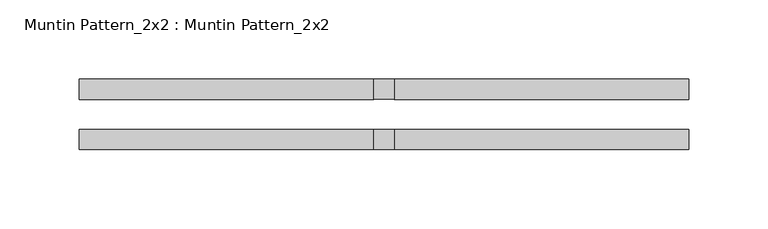
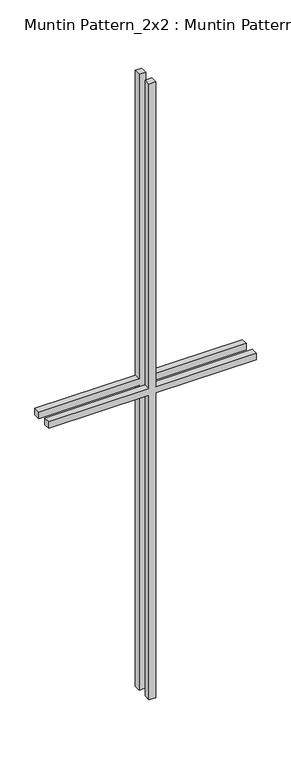
"""IFC4 building model written with IfcOpenShell, lengths in millimetres: proxy geometry, Muntin Pattern_2x2 : Muntin Pattern_2x2."""

from ifc_helpers import new_model, si_unit, frame, origin, place, context, project, spatial, polyline, outline, extrude, source, transform, mapped, element, save


def muntin_pattern_2x2_muntin_pattern_2x2_3dfd0a47(model_context):
    return source(origin(), model_context, "Body", "SweptSolid", [
        extrude(outline(polyline([(609.6, -6.35), (609.6, -192.0875), (596.9, -192.0875), (596.9, -6.35), (0.0, -6.35), (0.0, 6.35), (596.9, 6.35), (596.9, 192.0875), (609.6, 192.0875), (609.6, 6.35), (1206.5, 6.35), (1206.5, -6.35), (609.6, -6.35)])), frame((0.0, -22.225, 0.0), z_axis=(0.0, 1.0, 0.0), x_axis=(0.0, 0.0, 1.0)), (0.0, 0.0, 1.0), 12.7),
        extrude(outline(polyline([(609.6, -6.35), (609.6, -192.0875), (596.9, -192.0875), (596.9, -6.35), (0.0, -6.35), (0.0, 6.35), (596.9, 6.35), (596.9, 192.0875), (609.6, 192.0875), (609.6, 6.35), (1206.5, 6.35), (1206.5, -6.35), (609.6, -6.35)])), frame((0.0, 9.525, 0.0), z_axis=(0.0, 1.0, 0.0), x_axis=(0.0, 0.0, 1.0)), (0.0, 0.0, 1.0), 12.7),
    ])


if __name__ == "__main__":
    model = new_model("IFC4")
    model_context = context("Model", 3, world=origin())
    ifc_project = project(units=[si_unit("LENGTHUNIT", "METRE", prefix="MILLI")], contexts=[model_context])
    site = spatial("IfcSite", under=ifc_project)
    building = spatial("IfcBuilding", under=site)
    placement = place(None, origin())
    muntin_pattern_2x2_muntin_pattern_2x2_shape = muntin_pattern_2x2_muntin_pattern_2x2_3dfd0a47(model_context)
    element("IfcBuildingElementProxy", 1, Name="Muntin Pattern_2x2 : Muntin Pattern_2x2", ObjectType="Muntin Pattern_2x2 : Muntin Pattern_2x2", at=placement, inside=building, context=model_context, shape_type="MappedRepresentation", body=[
        mapped(muntin_pattern_2x2_muntin_pattern_2x2_shape, transform((0.0, 0.0, 0.0), x_axis=(1.0, 0.0, 0.0), y_axis=(0.0, 1.0, 0.0), z_axis=(0.0, 0.0, 1.0))),
    ])
    save(model, "model.ifc")

# Revit data of these elements
# Type "Muntin Pattern_2x2 : Muntin Pattern_2x2"
#   Width [instance default] = 4' - 0"
#   Thickness = 0' - 0 1/2"
#   Height [instance default] = 4' - 0"
#   Distance = 0' - 0 3/4"
#   Interior Material [instance default] = none
#   Exterior Material [instance default] = none
#   Default Elevation = 0
# Element 1 (IfcBuildingElementProxy, "Muntin Pattern_2x2 : Muntin Pattern_2x2")
#   Width = 1' - 3 1/8"
#   Height = 3' - 11 1/2"
#   Interior Material = Wood - Stained
#   Materials on its faces: "Wood - Stained"
# Materials
#   "Wood - Stained": class "Wood", colour RGB 224 178 126, transparency 0, Cost = 0
